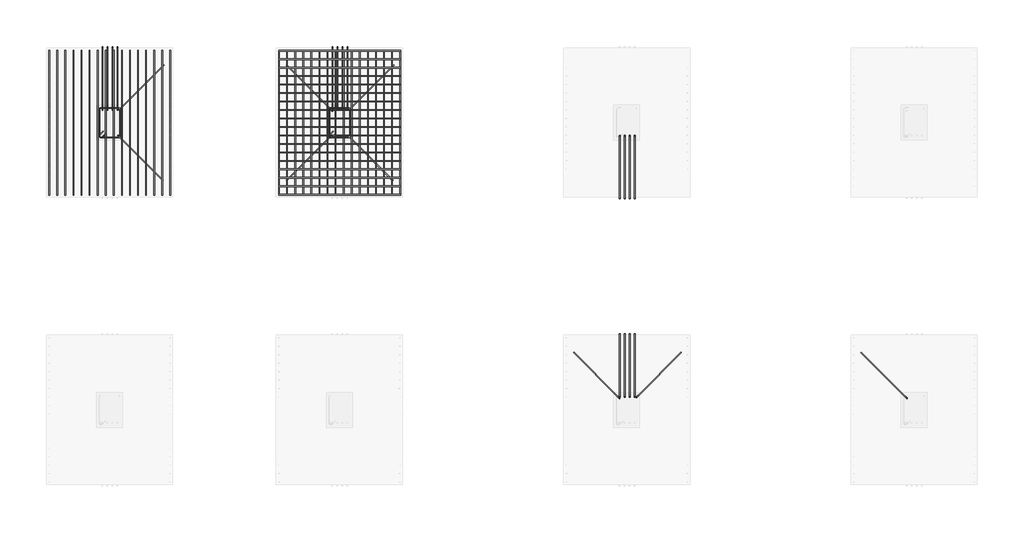
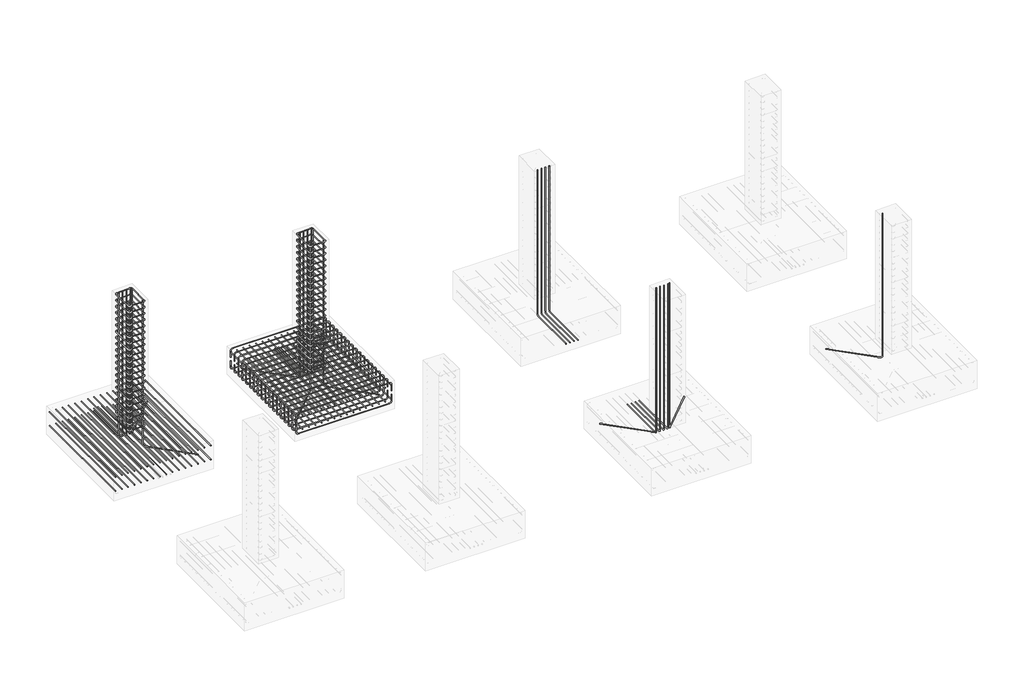
# One storey, part 5 of 33: 21 reinforcing bars.
"""IFC4 building model written with IfcOpenShell, lengths in millimetres."""

from ifc_helpers import new_model, si_unit, point, frame, origin, place, context, project, spatial, polyline, circle_curve, trimmed, segment, composite_curve, source, transform, mapped, element, save
from ifc_brep_helpers import swept_disk

model = new_model("IFC4")

# Units and contexts
model_context = context("Model", 3, world=origin())
ifc_project = project(units=[si_unit("LENGTHUNIT", "METRE", prefix="MILLI")], contexts=[model_context])

# Site, building, storey
site = spatial("IfcSite", under=ifc_project)
building = spatial("IfcBuilding", under=site)
storey = spatial("IfcBuildingStorey", under=building, Elevation=-3000.0)

# Reinforcing bars
placement = place(None, origin())
reinforcing_bar_shape = source(origin(), model_context, "Body", "SolidModel", [
    swept_disk(composite_curve([segment(polyline([(-10693.4642742, -2044.0608134, -3240.0), (-10693.4642742, -2044.0608134, -3092.7)]), True, "CONTINUOUS"), segment(trimmed(circle_curve(frame((-10647.1142742, -2044.0608134, -3092.7), z_axis=(0.0, 1.0, 0.0), x_axis=(-46.350000000000364, 0.0, 0.0)), 46.35), [point((-10693.4642742, -2044.0608134, -3092.7))], [point((-10647.1142742, -2044.0608134, -3046.35))], True, "CARTESIAN"), True, "CONTINUOUS"), segment(polyline([(-10647.1142742, -2044.0608134, -3046.35), (-8632.5142742, -2044.0608134, -3046.35)]), True, "CONTINUOUS"), segment(trimmed(circle_curve(frame((-8632.5142742, -2044.0608134, -3092.7), z_axis=(0.0, 1.0, 0.0), x_axis=(0.0, 0.0, 46.34999999999991)), 46.35), [point((-8632.5142742, -2044.0608134, -3046.35))], [point((-8586.1642742, -2044.0608134, -3092.7))], True, "CARTESIAN"), True, "CONTINUOUS"), segment(polyline([(-8586.1642742, -2044.0608134, -3092.7), (-8586.1642742, -2044.0608134, -3240.0)]), True, "CONTINUOUS")], self_intersect=False), 6.35),
])
element("IfcReinforcingBar", 1, at=placement, inside=storey, context=model_context, shape_type="MappedRepresentation", body=[
    mapped(reinforcing_bar_shape, transform((0.0, 0.0, 0.0), x_axis=(1.0, 0.0, 0.0), y_axis=(0.0, 1.0, 0.0), z_axis=(0.0, 0.0, 1.0))),
    mapped(reinforcing_bar_shape, transform((0.0, -147.4882353, 0.0), x_axis=(1.0, 0.0, 0.0), y_axis=(0.0, 1.0, 0.0), z_axis=(0.0, 0.0, 1.0))),
    mapped(reinforcing_bar_shape, transform((0.0, -294.9764706, 0.0), x_axis=(1.0, 0.0, 0.0), y_axis=(0.0, 1.0, 0.0), z_axis=(0.0, 0.0, 1.0))),
    mapped(reinforcing_bar_shape, transform((0.0, -442.4647059, 0.0), x_axis=(1.0, 0.0, 0.0), y_axis=(0.0, 1.0, 0.0), z_axis=(0.0, 0.0, 1.0))),
    mapped(reinforcing_bar_shape, transform((0.0, -589.9529412, 0.0), x_axis=(1.0, 0.0, 0.0), y_axis=(0.0, 1.0, 0.0), z_axis=(0.0, 0.0, 1.0))),
    mapped(reinforcing_bar_shape, transform((0.0, -737.4411765, 0.0), x_axis=(1.0, 0.0, 0.0), y_axis=(0.0, 1.0, 0.0), z_axis=(0.0, 0.0, 1.0))),
    mapped(reinforcing_bar_shape, transform((0.0, -884.9294118, 0.0), x_axis=(1.0, 0.0, 0.0), y_axis=(0.0, 1.0, 0.0), z_axis=(0.0, 0.0, 1.0))),
    mapped(reinforcing_bar_shape, transform((0.0, -1032.4176471, 0.0), x_axis=(1.0, 0.0, 0.0), y_axis=(0.0, 1.0, 0.0), z_axis=(0.0, 0.0, 1.0))),
    mapped(reinforcing_bar_shape, transform((0.0, -1179.9058824, 0.0), x_axis=(1.0, 0.0, 0.0), y_axis=(0.0, 1.0, 0.0), z_axis=(0.0, 0.0, 1.0))),
    mapped(reinforcing_bar_shape, transform((0.0, -1327.3941176, 0.0), x_axis=(1.0, 0.0, 0.0), y_axis=(0.0, 1.0, 0.0), z_axis=(0.0, 0.0, 1.0))),
    mapped(reinforcing_bar_shape, transform((0.0, -1474.8823529, 0.0), x_axis=(1.0, 0.0, 0.0), y_axis=(0.0, 1.0, 0.0), z_axis=(0.0, 0.0, 1.0))),
    mapped(reinforcing_bar_shape, transform((0.0, -1622.3705882, 0.0), x_axis=(1.0, 0.0, 0.0), y_axis=(0.0, 1.0, 0.0), z_axis=(0.0, 0.0, 1.0))),
    mapped(reinforcing_bar_shape, transform((0.0, -1769.8588235, 0.0), x_axis=(1.0, 0.0, 0.0), y_axis=(0.0, 1.0, 0.0), z_axis=(0.0, 0.0, 1.0))),
    mapped(reinforcing_bar_shape, transform((0.0, -1917.3470588, 0.0), x_axis=(1.0, 0.0, 0.0), y_axis=(0.0, 1.0, 0.0), z_axis=(0.0, 0.0, 1.0))),
    mapped(reinforcing_bar_shape, transform((0.0, -2064.8352941, 0.0), x_axis=(1.0, 0.0, 0.0), y_axis=(0.0, 1.0, 0.0), z_axis=(0.0, 0.0, 1.0))),
    mapped(reinforcing_bar_shape, transform((0.0, -2212.3235294, 0.0), x_axis=(1.0, 0.0, 0.0), y_axis=(0.0, 1.0, 0.0), z_axis=(0.0, 0.0, 1.0))),
    mapped(reinforcing_bar_shape, transform((0.0, -2359.8117647, 0.0), x_axis=(1.0, 0.0, 0.0), y_axis=(0.0, 1.0, 0.0), z_axis=(0.0, 0.0, 1.0))),
    mapped(reinforcing_bar_shape, transform((0.0, -2507.3, 0.0), x_axis=(1.0, 0.0, 0.0), y_axis=(0.0, 1.0, 0.0), z_axis=(0.0, 0.0, 1.0))),
])
reinforcing_bar_2_shape = source(origin(), model_context, "Body", "SolidModel", [
    swept_disk(composite_curve([segment(polyline([(-8586.1642742, -2044.0608134, -3330.080452), (-8586.1642742, -2044.0608134, -3477.380452)]), True, "CONTINUOUS"), segment(trimmed(circle_curve(frame((-8632.5142742, -2044.0608134, -3477.380452), z_axis=(0.0, 1.0, 0.0), x_axis=(46.350000000000364, 0.0, 0.0)), 46.35), [point((-8586.1642742, -2044.0608134, -3477.380452))], [point((-8632.5142742, -2044.0608134, -3523.730452))], True, "CARTESIAN"), True, "CONTINUOUS"), segment(polyline([(-8632.5142742, -2044.0608134, -3523.730452), (-10647.1142742, -2044.0608134, -3523.730452)]), True, "CONTINUOUS"), segment(trimmed(circle_curve(frame((-10647.1142742, -2044.0608134, -3477.380452), z_axis=(0.0, 1.0, 0.0), x_axis=(0.0, 0.0, -46.34999999999991)), 46.35), [point((-10647.1142742, -2044.0608134, -3523.730452))], [point((-10693.4642742, -2044.0608134, -3477.380452))], True, "CARTESIAN"), True, "CONTINUOUS"), segment(polyline([(-10693.4642742, -2044.0608134, -3477.380452), (-10693.4642742, -2044.0608134, -3330.080452)]), True, "CONTINUOUS")], self_intersect=False), 6.35),
])
element("IfcReinforcingBar", 2, at=placement, inside=storey, context=model_context, shape_type="MappedRepresentation", body=[
    mapped(reinforcing_bar_2_shape, transform((0.0, 0.0, 0.0), x_axis=(1.0, 0.0, 0.0), y_axis=(0.0, 1.0, 0.0), z_axis=(0.0, 0.0, 1.0))),
    mapped(reinforcing_bar_2_shape, transform((0.0, -147.4882353, 0.0), x_axis=(1.0, 0.0, 0.0), y_axis=(0.0, 1.0, 0.0), z_axis=(0.0, 0.0, 1.0))),
    mapped(reinforcing_bar_2_shape, transform((0.0, -294.9764706, 0.0), x_axis=(1.0, 0.0, 0.0), y_axis=(0.0, 1.0, 0.0), z_axis=(0.0, 0.0, 1.0))),
    mapped(reinforcing_bar_2_shape, transform((0.0, -442.4647059, 0.0), x_axis=(1.0, 0.0, 0.0), y_axis=(0.0, 1.0, 0.0), z_axis=(0.0, 0.0, 1.0))),
    mapped(reinforcing_bar_2_shape, transform((0.0, -589.9529412, 0.0), x_axis=(1.0, 0.0, 0.0), y_axis=(0.0, 1.0, 0.0), z_axis=(0.0, 0.0, 1.0))),
    mapped(reinforcing_bar_2_shape, transform((0.0, -737.4411765, 0.0), x_axis=(1.0, 0.0, 0.0), y_axis=(0.0, 1.0, 0.0), z_axis=(0.0, 0.0, 1.0))),
    mapped(reinforcing_bar_2_shape, transform((0.0, -884.9294118, 0.0), x_axis=(1.0, 0.0, 0.0), y_axis=(0.0, 1.0, 0.0), z_axis=(0.0, 0.0, 1.0))),
    mapped(reinforcing_bar_2_shape, transform((0.0, -1032.4176471, 0.0), x_axis=(1.0, 0.0, 0.0), y_axis=(0.0, 1.0, 0.0), z_axis=(0.0, 0.0, 1.0))),
    mapped(reinforcing_bar_2_shape, transform((0.0, -1179.9058824, 0.0), x_axis=(1.0, 0.0, 0.0), y_axis=(0.0, 1.0, 0.0), z_axis=(0.0, 0.0, 1.0))),
    mapped(reinforcing_bar_2_shape, transform((0.0, -1327.3941176, 0.0), x_axis=(1.0, 0.0, 0.0), y_axis=(0.0, 1.0, 0.0), z_axis=(0.0, 0.0, 1.0))),
    mapped(reinforcing_bar_2_shape, transform((0.0, -1474.8823529, 0.0), x_axis=(1.0, 0.0, 0.0), y_axis=(0.0, 1.0, 0.0), z_axis=(0.0, 0.0, 1.0))),
    mapped(reinforcing_bar_2_shape, transform((0.0, -1622.3705882, 0.0), x_axis=(1.0, 0.0, 0.0), y_axis=(0.0, 1.0, 0.0), z_axis=(0.0, 0.0, 1.0))),
    mapped(reinforcing_bar_2_shape, transform((0.0, -1769.8588235, 0.0), x_axis=(1.0, 0.0, 0.0), y_axis=(0.0, 1.0, 0.0), z_axis=(0.0, 0.0, 1.0))),
    mapped(reinforcing_bar_2_shape, transform((0.0, -1917.3470588, 0.0), x_axis=(1.0, 0.0, 0.0), y_axis=(0.0, 1.0, 0.0), z_axis=(0.0, 0.0, 1.0))),
    mapped(reinforcing_bar_2_shape, transform((0.0, -2064.8352941, 0.0), x_axis=(1.0, 0.0, 0.0), y_axis=(0.0, 1.0, 0.0), z_axis=(0.0, 0.0, 1.0))),
    mapped(reinforcing_bar_2_shape, transform((0.0, -2212.3235294, 0.0), x_axis=(1.0, 0.0, 0.0), y_axis=(0.0, 1.0, 0.0), z_axis=(0.0, 0.0, 1.0))),
    mapped(reinforcing_bar_2_shape, transform((0.0, -2359.8117647, 0.0), x_axis=(1.0, 0.0, 0.0), y_axis=(0.0, 1.0, 0.0), z_axis=(0.0, 0.0, 1.0))),
    mapped(reinforcing_bar_2_shape, transform((0.0, -2507.3, 0.0), x_axis=(1.0, 0.0, 0.0), y_axis=(0.0, 1.0, 0.0), z_axis=(0.0, 0.0, 1.0))),
])
reinforcing_bar_3_shape = source(origin(), model_context, "Body", "SolidModel", [
    swept_disk(composite_curve([segment(polyline([(-8586.1642742, -4557.7108134, -3447.8614173), (-8586.1642742, -2037.7108134, -3447.8614173)]), True, "CONTINUOUS")], self_intersect=False), 6.35),
])
element("IfcReinforcingBar", 3, at=placement, inside=storey, context=model_context, shape_type="MappedRepresentation", body=[
    mapped(reinforcing_bar_3_shape, transform((0.0, 0.0, 0.0), x_axis=(1.0, 0.0, 0.0), y_axis=(0.0, 1.0, 0.0), z_axis=(0.0, 0.0, 1.0))),
    mapped(reinforcing_bar_3_shape, transform((-140.4866667, 0.0, 0.0), x_axis=(1.0, 0.0, 0.0), y_axis=(0.0, 1.0, 0.0), z_axis=(0.0, 0.0, 1.0))),
    mapped(reinforcing_bar_3_shape, transform((-280.9733333, 0.0, 0.0), x_axis=(1.0, 0.0, 0.0), y_axis=(0.0, 1.0, 0.0), z_axis=(0.0, 0.0, 1.0))),
    mapped(reinforcing_bar_3_shape, transform((-421.46, 0.0, 0.0), x_axis=(1.0, 0.0, 0.0), y_axis=(0.0, 1.0, 0.0), z_axis=(0.0, 0.0, 1.0))),
    mapped(reinforcing_bar_3_shape, transform((-561.9466667, 0.0, 0.0), x_axis=(1.0, 0.0, 0.0), y_axis=(0.0, 1.0, 0.0), z_axis=(0.0, 0.0, 1.0))),
    mapped(reinforcing_bar_3_shape, transform((-702.4333333, 0.0, 0.0), x_axis=(1.0, 0.0, 0.0), y_axis=(0.0, 1.0, 0.0), z_axis=(0.0, 0.0, 1.0))),
    mapped(reinforcing_bar_3_shape, transform((-842.92, 0.0, 0.0), x_axis=(1.0, 0.0, 0.0), y_axis=(0.0, 1.0, 0.0), z_axis=(0.0, 0.0, 1.0))),
    mapped(reinforcing_bar_3_shape, transform((-983.4066667, 0.0, 0.0), x_axis=(1.0, 0.0, 0.0), y_axis=(0.0, 1.0, 0.0), z_axis=(0.0, 0.0, 1.0))),
    mapped(reinforcing_bar_3_shape, transform((-1123.8933333, 0.0, 0.0), x_axis=(1.0, 0.0, 0.0), y_axis=(0.0, 1.0, 0.0), z_axis=(0.0, 0.0, 1.0))),
    mapped(reinforcing_bar_3_shape, transform((-1264.38, 0.0, 0.0), x_axis=(1.0, 0.0, 0.0), y_axis=(0.0, 1.0, 0.0), z_axis=(0.0, 0.0, 1.0))),
    mapped(reinforcing_bar_3_shape, transform((-1404.8666667, 0.0, 0.0), x_axis=(1.0, 0.0, 0.0), y_axis=(0.0, 1.0, 0.0), z_axis=(0.0, 0.0, 1.0))),
    mapped(reinforcing_bar_3_shape, transform((-1545.3533333, 0.0, 0.0), x_axis=(1.0, 0.0, 0.0), y_axis=(0.0, 1.0, 0.0), z_axis=(0.0, 0.0, 1.0))),
    mapped(reinforcing_bar_3_shape, transform((-1685.84, 0.0, 0.0), x_axis=(1.0, 0.0, 0.0), y_axis=(0.0, 1.0, 0.0), z_axis=(0.0, 0.0, 1.0))),
    mapped(reinforcing_bar_3_shape, transform((-1826.3266667, 0.0, 0.0), x_axis=(1.0, 0.0, 0.0), y_axis=(0.0, 1.0, 0.0), z_axis=(0.0, 0.0, 1.0))),
    mapped(reinforcing_bar_3_shape, transform((-1966.8133333, 0.0, 0.0), x_axis=(1.0, 0.0, 0.0), y_axis=(0.0, 1.0, 0.0), z_axis=(0.0, 0.0, 1.0))),
    mapped(reinforcing_bar_3_shape, transform((-2107.3, 0.0, 0.0), x_axis=(1.0, 0.0, 0.0), y_axis=(0.0, 1.0, 0.0), z_axis=(0.0, 0.0, 1.0))),
])
reinforcing_bar_4_shape = source(origin(), model_context, "Body", "SolidModel", [
    swept_disk(composite_curve([segment(polyline([(-10693.4642742, -4557.7108134, -3122.7084113), (-10693.4642742, -2037.7108134, -3122.7084113)]), True, "CONTINUOUS")], self_intersect=False), 6.35),
])
element("IfcReinforcingBar", 4, at=placement, inside=storey, context=model_context, shape_type="MappedRepresentation", body=[
    mapped(reinforcing_bar_4_shape, transform((0.0, 0.0, 0.0), x_axis=(1.0, 0.0, 0.0), y_axis=(0.0, 1.0, 0.0), z_axis=(0.0, 0.0, 1.0))),
    mapped(reinforcing_bar_4_shape, transform((140.4866667, 0.0, 0.0), x_axis=(1.0, 0.0, 0.0), y_axis=(0.0, 1.0, 0.0), z_axis=(0.0, 0.0, 1.0))),
    mapped(reinforcing_bar_4_shape, transform((280.9733333, 0.0, 0.0), x_axis=(1.0, 0.0, 0.0), y_axis=(0.0, 1.0, 0.0), z_axis=(0.0, 0.0, 1.0))),
    mapped(reinforcing_bar_4_shape, transform((421.46, 0.0, 0.0), x_axis=(1.0, 0.0, 0.0), y_axis=(0.0, 1.0, 0.0), z_axis=(0.0, 0.0, 1.0))),
    mapped(reinforcing_bar_4_shape, transform((561.9466667, 0.0, 0.0), x_axis=(1.0, 0.0, 0.0), y_axis=(0.0, 1.0, 0.0), z_axis=(0.0, 0.0, 1.0))),
    mapped(reinforcing_bar_4_shape, transform((702.4333333, 0.0, 0.0), x_axis=(1.0, 0.0, 0.0), y_axis=(0.0, 1.0, 0.0), z_axis=(0.0, 0.0, 1.0))),
    mapped(reinforcing_bar_4_shape, transform((842.92, 0.0, 0.0), x_axis=(1.0, 0.0, 0.0), y_axis=(0.0, 1.0, 0.0), z_axis=(0.0, 0.0, 1.0))),
    mapped(reinforcing_bar_4_shape, transform((983.4066667, 0.0, 0.0), x_axis=(1.0, 0.0, 0.0), y_axis=(0.0, 1.0, 0.0), z_axis=(0.0, 0.0, 1.0))),
    mapped(reinforcing_bar_4_shape, transform((1123.8933333, 0.0, 0.0), x_axis=(1.0, 0.0, 0.0), y_axis=(0.0, 1.0, 0.0), z_axis=(0.0, 0.0, 1.0))),
    mapped(reinforcing_bar_4_shape, transform((1264.38, 0.0, 0.0), x_axis=(1.0, 0.0, 0.0), y_axis=(0.0, 1.0, 0.0), z_axis=(0.0, 0.0, 1.0))),
    mapped(reinforcing_bar_4_shape, transform((1404.8666667, 0.0, 0.0), x_axis=(1.0, 0.0, 0.0), y_axis=(0.0, 1.0, 0.0), z_axis=(0.0, 0.0, 1.0))),
    mapped(reinforcing_bar_4_shape, transform((1545.3533333, 0.0, 0.0), x_axis=(1.0, 0.0, 0.0), y_axis=(0.0, 1.0, 0.0), z_axis=(0.0, 0.0, 1.0))),
    mapped(reinforcing_bar_4_shape, transform((1685.84, 0.0, 0.0), x_axis=(1.0, 0.0, 0.0), y_axis=(0.0, 1.0, 0.0), z_axis=(0.0, 0.0, 1.0))),
    mapped(reinforcing_bar_4_shape, transform((1826.3266667, 0.0, 0.0), x_axis=(1.0, 0.0, 0.0), y_axis=(0.0, 1.0, 0.0), z_axis=(0.0, 0.0, 1.0))),
    mapped(reinforcing_bar_4_shape, transform((1966.8133333, 0.0, 0.0), x_axis=(1.0, 0.0, 0.0), y_axis=(0.0, 1.0, 0.0), z_axis=(0.0, 0.0, 1.0))),
    mapped(reinforcing_bar_4_shape, transform((2107.3, 0.0, 0.0), x_axis=(1.0, 0.0, 0.0), y_axis=(0.0, 1.0, 0.0), z_axis=(0.0, 0.0, 1.0))),
])
reinforcing_bar_5_shape = source(origin(), model_context, "Body", "SolidModel", [
    swept_disk(composite_curve([segment(polyline([(-12586.1642742, -4557.7108134, -3447.8614173), (-12586.1642742, -2037.7108134, -3447.8614173)]), True, "CONTINUOUS")], self_intersect=False), 6.35),
])
element("IfcReinforcingBar", 5, at=placement, inside=storey, context=model_context, shape_type="MappedRepresentation", body=[
    mapped(reinforcing_bar_5_shape, transform((0.0, 0.0, 0.0), x_axis=(1.0, 0.0, 0.0), y_axis=(0.0, 1.0, 0.0), z_axis=(0.0, 0.0, 1.0))),
    mapped(reinforcing_bar_5_shape, transform((-140.4866667, 0.0, 0.0), x_axis=(1.0, 0.0, 0.0), y_axis=(0.0, 1.0, 0.0), z_axis=(0.0, 0.0, 1.0))),
    mapped(reinforcing_bar_5_shape, transform((-280.9733333, 0.0, 0.0), x_axis=(1.0, 0.0, 0.0), y_axis=(0.0, 1.0, 0.0), z_axis=(0.0, 0.0, 1.0))),
    mapped(reinforcing_bar_5_shape, transform((-421.46, 0.0, 0.0), x_axis=(1.0, 0.0, 0.0), y_axis=(0.0, 1.0, 0.0), z_axis=(0.0, 0.0, 1.0))),
    mapped(reinforcing_bar_5_shape, transform((-561.9466667, 0.0, 0.0), x_axis=(1.0, 0.0, 0.0), y_axis=(0.0, 1.0, 0.0), z_axis=(0.0, 0.0, 1.0))),
    mapped(reinforcing_bar_5_shape, transform((-702.4333333, 0.0, 0.0), x_axis=(1.0, 0.0, 0.0), y_axis=(0.0, 1.0, 0.0), z_axis=(0.0, 0.0, 1.0))),
    mapped(reinforcing_bar_5_shape, transform((-842.92, 0.0, 0.0), x_axis=(1.0, 0.0, 0.0), y_axis=(0.0, 1.0, 0.0), z_axis=(0.0, 0.0, 1.0))),
    mapped(reinforcing_bar_5_shape, transform((-983.4066667, 0.0, 0.0), x_axis=(1.0, 0.0, 0.0), y_axis=(0.0, 1.0, 0.0), z_axis=(0.0, 0.0, 1.0))),
    mapped(reinforcing_bar_5_shape, transform((-1123.8933333, 0.0, 0.0), x_axis=(1.0, 0.0, 0.0), y_axis=(0.0, 1.0, 0.0), z_axis=(0.0, 0.0, 1.0))),
    mapped(reinforcing_bar_5_shape, transform((-1264.38, 0.0, 0.0), x_axis=(1.0, 0.0, 0.0), y_axis=(0.0, 1.0, 0.0), z_axis=(0.0, 0.0, 1.0))),
    mapped(reinforcing_bar_5_shape, transform((-1404.8666667, 0.0, 0.0), x_axis=(1.0, 0.0, 0.0), y_axis=(0.0, 1.0, 0.0), z_axis=(0.0, 0.0, 1.0))),
    mapped(reinforcing_bar_5_shape, transform((-1545.3533333, 0.0, 0.0), x_axis=(1.0, 0.0, 0.0), y_axis=(0.0, 1.0, 0.0), z_axis=(0.0, 0.0, 1.0))),
    mapped(reinforcing_bar_5_shape, transform((-1685.84, 0.0, 0.0), x_axis=(1.0, 0.0, 0.0), y_axis=(0.0, 1.0, 0.0), z_axis=(0.0, 0.0, 1.0))),
    mapped(reinforcing_bar_5_shape, transform((-1826.3266667, 0.0, 0.0), x_axis=(1.0, 0.0, 0.0), y_axis=(0.0, 1.0, 0.0), z_axis=(0.0, 0.0, 1.0))),
    mapped(reinforcing_bar_5_shape, transform((-1966.8133333, 0.0, 0.0), x_axis=(1.0, 0.0, 0.0), y_axis=(0.0, 1.0, 0.0), z_axis=(0.0, 0.0, 1.0))),
    mapped(reinforcing_bar_5_shape, transform((-2107.3, 0.0, 0.0), x_axis=(1.0, 0.0, 0.0), y_axis=(0.0, 1.0, 0.0), z_axis=(0.0, 0.0, 1.0))),
])
reinforcing_bar_6_shape = source(origin(), model_context, "Body", "SolidModel", [
    swept_disk(composite_curve([segment(polyline([(-14693.4642742, -4557.7108134, -3122.7084113), (-14693.4642742, -2037.7108134, -3122.7084113)]), True, "CONTINUOUS")], self_intersect=False), 6.35),
])
element("IfcReinforcingBar", 6, at=placement, inside=storey, context=model_context, shape_type="MappedRepresentation", body=[
    mapped(reinforcing_bar_6_shape, transform((0.0, 0.0, 0.0), x_axis=(1.0, 0.0, 0.0), y_axis=(0.0, 1.0, 0.0), z_axis=(0.0, 0.0, 1.0))),
    mapped(reinforcing_bar_6_shape, transform((140.4866667, 0.0, 0.0), x_axis=(1.0, 0.0, 0.0), y_axis=(0.0, 1.0, 0.0), z_axis=(0.0, 0.0, 1.0))),
    mapped(reinforcing_bar_6_shape, transform((280.9733333, 0.0, 0.0), x_axis=(1.0, 0.0, 0.0), y_axis=(0.0, 1.0, 0.0), z_axis=(0.0, 0.0, 1.0))),
    mapped(reinforcing_bar_6_shape, transform((421.46, 0.0, 0.0), x_axis=(1.0, 0.0, 0.0), y_axis=(0.0, 1.0, 0.0), z_axis=(0.0, 0.0, 1.0))),
    mapped(reinforcing_bar_6_shape, transform((561.9466667, 0.0, 0.0), x_axis=(1.0, 0.0, 0.0), y_axis=(0.0, 1.0, 0.0), z_axis=(0.0, 0.0, 1.0))),
    mapped(reinforcing_bar_6_shape, transform((702.4333333, 0.0, 0.0), x_axis=(1.0, 0.0, 0.0), y_axis=(0.0, 1.0, 0.0), z_axis=(0.0, 0.0, 1.0))),
    mapped(reinforcing_bar_6_shape, transform((842.92, 0.0, 0.0), x_axis=(1.0, 0.0, 0.0), y_axis=(0.0, 1.0, 0.0), z_axis=(0.0, 0.0, 1.0))),
    mapped(reinforcing_bar_6_shape, transform((983.4066667, 0.0, 0.0), x_axis=(1.0, 0.0, 0.0), y_axis=(0.0, 1.0, 0.0), z_axis=(0.0, 0.0, 1.0))),
    mapped(reinforcing_bar_6_shape, transform((1123.8933333, 0.0, 0.0), x_axis=(1.0, 0.0, 0.0), y_axis=(0.0, 1.0, 0.0), z_axis=(0.0, 0.0, 1.0))),
    mapped(reinforcing_bar_6_shape, transform((1264.38, 0.0, 0.0), x_axis=(1.0, 0.0, 0.0), y_axis=(0.0, 1.0, 0.0), z_axis=(0.0, 0.0, 1.0))),
    mapped(reinforcing_bar_6_shape, transform((1404.8666667, 0.0, 0.0), x_axis=(1.0, 0.0, 0.0), y_axis=(0.0, 1.0, 0.0), z_axis=(0.0, 0.0, 1.0))),
    mapped(reinforcing_bar_6_shape, transform((1545.3533333, 0.0, 0.0), x_axis=(1.0, 0.0, 0.0), y_axis=(0.0, 1.0, 0.0), z_axis=(0.0, 0.0, 1.0))),
    mapped(reinforcing_bar_6_shape, transform((1685.84, 0.0, 0.0), x_axis=(1.0, 0.0, 0.0), y_axis=(0.0, 1.0, 0.0), z_axis=(0.0, 0.0, 1.0))),
    mapped(reinforcing_bar_6_shape, transform((1826.3266667, 0.0, 0.0), x_axis=(1.0, 0.0, 0.0), y_axis=(0.0, 1.0, 0.0), z_axis=(0.0, 0.0, 1.0))),
    mapped(reinforcing_bar_6_shape, transform((1966.8133333, 0.0, 0.0), x_axis=(1.0, 0.0, 0.0), y_axis=(0.0, 1.0, 0.0), z_axis=(0.0, 0.0, 1.0))),
    mapped(reinforcing_bar_6_shape, transform((2107.3, 0.0, 0.0), x_axis=(1.0, 0.0, 0.0), y_axis=(0.0, 1.0, 0.0), z_axis=(0.0, 0.0, 1.0))),
])
reinforcing_bar_7_shape = source(origin(), model_context, "Body", "SolidModel", [
    swept_disk(composite_curve([segment(polyline([(-13753.5385089, -3446.8994528, -2953.65), (-13809.2820718, -3502.6430158, -2953.65)]), True, "CONTINUOUS"), segment(trimmed(circle_curve(frame((-13787.1142742, -3524.8108134, -2953.65), z_axis=(0.0, 0.0, 1.0), x_axis=(-22.167797600000995, 22.167797600000085, 0.0)), 31.35), [point((-13809.2820718, -3502.6430158, -2953.65))], [point((-13787.1142742, -3556.1608134, -2953.65))], True, "CARTESIAN"), True, "CONTINUOUS"), segment(polyline([(-13787.1142742, -3556.1608134, -2953.65), (-13492.5142742, -3556.1608134, -2953.65)]), True, "CONTINUOUS"), segment(trimmed(circle_curve(frame((-13492.5142742, -3524.8108134, -2953.65), z_axis=(0.0, 0.0, 1.0), x_axis=(0.0, -31.34999999999991, 0.0)), 31.35), [point((-13492.5142742, -3556.1608134, -2953.65))], [point((-13461.1642742, -3524.8108134, -2953.65))], True, "CARTESIAN"), True, "CONTINUOUS"), segment(polyline([(-13461.1642742, -3524.8108134, -2953.65), (-13461.1642742, -3070.6108134, -2953.65)]), True, "CONTINUOUS"), segment(trimmed(circle_curve(frame((-13492.4944891, -3070.6108134, -2954.7636125), z_axis=(-0.0355219283344822, 0.0, 0.9993688971583016), x_axis=(31.33021489999919, 0.0, 1.1136124999998174)), 31.35), [point((-13461.1642742, -3070.6108134, -2953.65))], [point((-13492.4944891, -3039.2608134, -2954.7636125))], True, "CARTESIAN"), True, "CONTINUOUS"), segment(polyline([(-13492.4944891, -3039.2608134, -2954.7636125), (-13787.1340593, -3039.2608134, -2965.2363875)]), True, "CONTINUOUS"), segment(trimmed(circle_curve(frame((-13787.1340593, -3070.6108134, -2965.2363875), z_axis=(-0.0355219283344822, 0.0, 0.9993688971583016), x_axis=(0.0, 31.34999999999991, 0.0)), 31.35), [point((-13787.1340593, -3039.2608134, -2965.2363875))], [point((-13818.4642742, -3070.6108134, -2966.35))], True, "CARTESIAN"), True, "CONTINUOUS"), segment(polyline([(-13818.4642742, -3070.6108134, -2966.35), (-13818.4642742, -3524.8108134, -2966.35)]), True, "CONTINUOUS"), segment(trimmed(circle_curve(frame((-13787.1142742, -3524.8108134, -2966.35), z_axis=(0.0, 0.0, 1.0), x_axis=(-31.350000000000364, 0.0, 0.0)), 31.35), [point((-13818.4642742, -3524.8108134, -2966.35))], [point((-13764.9464766, -3546.978611, -2966.35))], True, "CARTESIAN"), True, "CONTINUOUS"), segment(polyline([(-13764.9464766, -3546.978611, -2966.35), (-13709.2029137, -3491.235048, -2966.35)]), True, "CONTINUOUS")], self_intersect=False), 6.35),
])
element("IfcReinforcingBar", 7, at=placement, inside=storey, context=model_context, shape_type="MappedRepresentation", body=[
    mapped(reinforcing_bar_7_shape, transform((0.0, 0.0, 0.0), x_axis=(1.0, 0.0, 0.0), y_axis=(0.0, 1.0, 0.0), z_axis=(0.0, 0.0, 1.0))),
    mapped(reinforcing_bar_7_shape, transform((0.0, 0.0, 145.365), x_axis=(1.0, 0.0, 0.0), y_axis=(0.0, 1.0, 0.0), z_axis=(0.0, 0.0, 1.0))),
    mapped(reinforcing_bar_7_shape, transform((0.0, 0.0, 290.73), x_axis=(1.0, 0.0, 0.0), y_axis=(0.0, 1.0, 0.0), z_axis=(0.0, 0.0, 1.0))),
    mapped(reinforcing_bar_7_shape, transform((0.0, 0.0, 436.095), x_axis=(1.0, 0.0, 0.0), y_axis=(0.0, 1.0, 0.0), z_axis=(0.0, 0.0, 1.0))),
    mapped(reinforcing_bar_7_shape, transform((0.0, 0.0, 581.46), x_axis=(1.0, 0.0, 0.0), y_axis=(0.0, 1.0, 0.0), z_axis=(0.0, 0.0, 1.0))),
    mapped(reinforcing_bar_7_shape, transform((0.0, 0.0, 726.825), x_axis=(1.0, 0.0, 0.0), y_axis=(0.0, 1.0, 0.0), z_axis=(0.0, 0.0, 1.0))),
    mapped(reinforcing_bar_7_shape, transform((0.0, 0.0, 872.19), x_axis=(1.0, 0.0, 0.0), y_axis=(0.0, 1.0, 0.0), z_axis=(0.0, 0.0, 1.0))),
    mapped(reinforcing_bar_7_shape, transform((0.0, 0.0, 1017.555), x_axis=(1.0, 0.0, 0.0), y_axis=(0.0, 1.0, 0.0), z_axis=(0.0, 0.0, 1.0))),
    mapped(reinforcing_bar_7_shape, transform((0.0, 0.0, 1162.92), x_axis=(1.0, 0.0, 0.0), y_axis=(0.0, 1.0, 0.0), z_axis=(0.0, 0.0, 1.0))),
    mapped(reinforcing_bar_7_shape, transform((0.0, 0.0, 1308.285), x_axis=(1.0, 0.0, 0.0), y_axis=(0.0, 1.0, 0.0), z_axis=(0.0, 0.0, 1.0))),
    mapped(reinforcing_bar_7_shape, transform((0.0, 0.0, 1453.65), x_axis=(1.0, 0.0, 0.0), y_axis=(0.0, 1.0, 0.0), z_axis=(0.0, 0.0, 1.0))),
    mapped(reinforcing_bar_7_shape, transform((0.0, 0.0, 1599.015), x_axis=(1.0, 0.0, 0.0), y_axis=(0.0, 1.0, 0.0), z_axis=(0.0, 0.0, 1.0))),
    mapped(reinforcing_bar_7_shape, transform((0.0, 0.0, 1744.38), x_axis=(1.0, 0.0, 0.0), y_axis=(0.0, 1.0, 0.0), z_axis=(0.0, 0.0, 1.0))),
    mapped(reinforcing_bar_7_shape, transform((0.0, 0.0, 1889.745), x_axis=(1.0, 0.0, 0.0), y_axis=(0.0, 1.0, 0.0), z_axis=(0.0, 0.0, 1.0))),
    mapped(reinforcing_bar_7_shape, transform((0.0, 0.0, 2035.11), x_axis=(1.0, 0.0, 0.0), y_axis=(0.0, 1.0, 0.0), z_axis=(0.0, 0.0, 1.0))),
    mapped(reinforcing_bar_7_shape, transform((0.0, 0.0, 2180.475), x_axis=(1.0, 0.0, 0.0), y_axis=(0.0, 1.0, 0.0), z_axis=(0.0, 0.0, 1.0))),
    mapped(reinforcing_bar_7_shape, transform((0.0, 0.0, 2325.84), x_axis=(1.0, 0.0, 0.0), y_axis=(0.0, 1.0, 0.0), z_axis=(0.0, 0.0, 1.0))),
    mapped(reinforcing_bar_7_shape, transform((0.0, 0.0, 2471.205), x_axis=(1.0, 0.0, 0.0), y_axis=(0.0, 1.0, 0.0), z_axis=(0.0, 0.0, 1.0))),
    mapped(reinforcing_bar_7_shape, transform((0.0, 0.0, 2616.57), x_axis=(1.0, 0.0, 0.0), y_axis=(0.0, 1.0, 0.0), z_axis=(0.0, 0.0, 1.0))),
    mapped(reinforcing_bar_7_shape, transform((0.0, 0.0, 2761.935), x_axis=(1.0, 0.0, 0.0), y_axis=(0.0, 1.0, 0.0), z_axis=(0.0, 0.0, 1.0))),
    mapped(reinforcing_bar_7_shape, transform((0.0, 0.0, 2907.3), x_axis=(1.0, 0.0, 0.0), y_axis=(0.0, 1.0, 0.0), z_axis=(0.0, 0.0, 1.0))),
])
element("IfcReinforcingBar", 8, at=placement, inside=storey, context=model_context, shape_type="SolidModel", body=[
    swept_disk(composite_curve([segment(polyline([(-13492.8328699, -3521.6339414, -40.0), (-13492.8328699, -3521.6339414, -3393.65)]), True, "CONTINUOUS"), segment(trimmed(circle_curve(frame((-13460.0584706, -3554.4083407, -3393.65), z_axis=(-0.7071067811865493, -0.7071067811865459, 0.0), x_axis=(-32.77439929999855, 32.774399299999914, 0.0)), 46.35), [point((-13492.8328699, -3521.6339414, -3393.65))], [point((-13460.0584706, -3554.4083407, -3440.0))], True, "CARTESIAN"), True, "CONTINUOUS"), segment(polyline([(-13460.0584706, -3554.4083407, -3440.0), (-12715.0154106, -4299.4514007, -3440.0)]), True, "CONTINUOUS")], self_intersect=False), 6.35),
])
element("IfcReinforcingBar", 9, at=placement, inside=storey, context=model_context, shape_type="SolidModel", body=[
    swept_disk(composite_curve([segment(polyline([(-13474.2315783, -3073.7876853, -30.2564663), (-13474.2315783, -3073.7876853, -3383.9064663)]), True, "CONTINUOUS"), segment(trimmed(circle_curve(frame((-13441.457179, -3041.013286, -3383.9064663), z_axis=(0.7071067811865493, -0.7071067811865459, 0.0), x_axis=(-32.77439929999855, -32.774399299999914, 0.0)), 46.35), [point((-13474.2315783, -3073.7876853, -3383.9064663))], [point((-13441.457179, -3041.013286, -3430.2564663))], True, "CARTESIAN"), True, "CONTINUOUS"), segment(polyline([(-13441.457179, -3041.013286, -3430.2564663), (-12696.414119, -2295.970226, -3430.2564663)]), True, "CONTINUOUS")], self_intersect=False), 6.35),
])
reinforcing_bar_8_shape = source(origin(), model_context, "Body", "SolidModel", [
    swept_disk(composite_curve([segment(polyline([(-13763.8841678, -3071.9278134, -40.0), (-13763.8841678, -3071.9278134, -3393.65)]), True, "CONTINUOUS"), segment(trimmed(circle_curve(frame((-13763.8841678, -3025.5778134, -3393.65), z_axis=(1.0, 0.0, 0.0), x_axis=(0.0, -46.34999999999991, 0.0)), 46.35), [point((-13763.8841678, -3071.9278134, -3393.65))], [point((-13763.8841678, -3025.5778134, -3440.0))], True, "CARTESIAN"), True, "CONTINUOUS"), segment(polyline([(-13763.8841678, -3025.5778134, -3440.0), (-13763.8841678, -1971.9278134, -3440.0)]), True, "CONTINUOUS")], self_intersect=False), 6.35),
])
element("IfcReinforcingBar", 10, at=placement, inside=storey, context=model_context, shape_type="MappedRepresentation", body=[
    mapped(reinforcing_bar_8_shape, transform((0.0, 0.0, 0.0), x_axis=(1.0, 0.0, 0.0), y_axis=(0.0, 1.0, 0.0), z_axis=(0.0, 0.0, 1.0))),
    mapped(reinforcing_bar_8_shape, transform((86.8979716, 0.0, 0.0), x_axis=(1.0, 0.0, 0.0), y_axis=(0.0, 1.0, 0.0), z_axis=(0.0, 0.0, 1.0))),
    mapped(reinforcing_bar_8_shape, transform((173.7959432, 0.0, 0.0), x_axis=(1.0, 0.0, 0.0), y_axis=(0.0, 1.0, 0.0), z_axis=(0.0, 0.0, 1.0))),
    mapped(reinforcing_bar_8_shape, transform((260.6939148, 0.0, 0.0), x_axis=(1.0, 0.0, 0.0), y_axis=(0.0, 1.0, 0.0), z_axis=(0.0, 0.0, 1.0))),
])
reinforcing_bar_9_shape = source(origin(), model_context, "Body", "SolidModel", [
    swept_disk(composite_curve([segment(polyline([(-9753.5385089, -3446.8994528, -2953.65), (-9809.2820718, -3502.6430158, -2953.65)]), True, "CONTINUOUS"), segment(trimmed(circle_curve(frame((-9787.1142742, -3524.8108134, -2953.65), z_axis=(0.0, 0.0, 1.0), x_axis=(-22.167797600000995, 22.167797600000085, 0.0)), 31.35), [point((-9809.2820718, -3502.6430158, -2953.65))], [point((-9787.1142742, -3556.1608134, -2953.65))], True, "CARTESIAN"), True, "CONTINUOUS"), segment(polyline([(-9787.1142742, -3556.1608134, -2953.65), (-9492.5142742, -3556.1608134, -2953.65)]), True, "CONTINUOUS"), segment(trimmed(circle_curve(frame((-9492.5142742, -3524.8108134, -2953.65), z_axis=(0.0, 0.0, 1.0), x_axis=(0.0, -31.34999999999991, 0.0)), 31.35), [point((-9492.5142742, -3556.1608134, -2953.65))], [point((-9461.1642742, -3524.8108134, -2953.65))], True, "CARTESIAN"), True, "CONTINUOUS"), segment(polyline([(-9461.1642742, -3524.8108134, -2953.65), (-9461.1642742, -3070.6108134, -2953.65)]), True, "CONTINUOUS"), segment(trimmed(circle_curve(frame((-9492.4944891, -3070.6108134, -2954.7636125), z_axis=(-0.0355219283344822, 0.0, 0.9993688971583016), x_axis=(31.33021489999919, 0.0, 1.1136124999998174)), 31.35), [point((-9461.1642742, -3070.6108134, -2953.65))], [point((-9492.4944891, -3039.2608134, -2954.7636125))], True, "CARTESIAN"), True, "CONTINUOUS"), segment(polyline([(-9492.4944891, -3039.2608134, -2954.7636125), (-9787.1340593, -3039.2608134, -2965.2363875)]), True, "CONTINUOUS"), segment(trimmed(circle_curve(frame((-9787.1340593, -3070.6108134, -2965.2363875), z_axis=(-0.0355219283344822, 0.0, 0.9993688971583016), x_axis=(0.0, 31.34999999999991, 0.0)), 31.35), [point((-9787.1340593, -3039.2608134, -2965.2363875))], [point((-9818.4642742, -3070.6108134, -2966.35))], True, "CARTESIAN"), True, "CONTINUOUS"), segment(polyline([(-9818.4642742, -3070.6108134, -2966.35), (-9818.4642742, -3524.8108134, -2966.35)]), True, "CONTINUOUS"), segment(trimmed(circle_curve(frame((-9787.1142742, -3524.8108134, -2966.35), z_axis=(0.0, 0.0, 1.0), x_axis=(-31.350000000000364, 0.0, 0.0)), 31.35), [point((-9818.4642742, -3524.8108134, -2966.35))], [point((-9764.9464766, -3546.978611, -2966.35))], True, "CARTESIAN"), True, "CONTINUOUS"), segment(polyline([(-9764.9464766, -3546.978611, -2966.35), (-9709.2029137, -3491.235048, -2966.35)]), True, "CONTINUOUS")], self_intersect=False), 6.35),
])
element("IfcReinforcingBar", 11, at=placement, inside=storey, context=model_context, shape_type="MappedRepresentation", body=[
    mapped(reinforcing_bar_9_shape, transform((0.0, 0.0, 0.0), x_axis=(1.0, 0.0, 0.0), y_axis=(0.0, 1.0, 0.0), z_axis=(0.0, 0.0, 1.0))),
    mapped(reinforcing_bar_9_shape, transform((0.0, 0.0, 145.365), x_axis=(1.0, 0.0, 0.0), y_axis=(0.0, 1.0, 0.0), z_axis=(0.0, 0.0, 1.0))),
    mapped(reinforcing_bar_9_shape, transform((0.0, 0.0, 290.73), x_axis=(1.0, 0.0, 0.0), y_axis=(0.0, 1.0, 0.0), z_axis=(0.0, 0.0, 1.0))),
    mapped(reinforcing_bar_9_shape, transform((0.0, 0.0, 436.095), x_axis=(1.0, 0.0, 0.0), y_axis=(0.0, 1.0, 0.0), z_axis=(0.0, 0.0, 1.0))),
    mapped(reinforcing_bar_9_shape, transform((0.0, 0.0, 581.46), x_axis=(1.0, 0.0, 0.0), y_axis=(0.0, 1.0, 0.0), z_axis=(0.0, 0.0, 1.0))),
    mapped(reinforcing_bar_9_shape, transform((0.0, 0.0, 726.825), x_axis=(1.0, 0.0, 0.0), y_axis=(0.0, 1.0, 0.0), z_axis=(0.0, 0.0, 1.0))),
    mapped(reinforcing_bar_9_shape, transform((0.0, 0.0, 872.19), x_axis=(1.0, 0.0, 0.0), y_axis=(0.0, 1.0, 0.0), z_axis=(0.0, 0.0, 1.0))),
    mapped(reinforcing_bar_9_shape, transform((0.0, 0.0, 1017.555), x_axis=(1.0, 0.0, 0.0), y_axis=(0.0, 1.0, 0.0), z_axis=(0.0, 0.0, 1.0))),
    mapped(reinforcing_bar_9_shape, transform((0.0, 0.0, 1162.92), x_axis=(1.0, 0.0, 0.0), y_axis=(0.0, 1.0, 0.0), z_axis=(0.0, 0.0, 1.0))),
    mapped(reinforcing_bar_9_shape, transform((0.0, 0.0, 1308.285), x_axis=(1.0, 0.0, 0.0), y_axis=(0.0, 1.0, 0.0), z_axis=(0.0, 0.0, 1.0))),
    mapped(reinforcing_bar_9_shape, transform((0.0, 0.0, 1453.65), x_axis=(1.0, 0.0, 0.0), y_axis=(0.0, 1.0, 0.0), z_axis=(0.0, 0.0, 1.0))),
    mapped(reinforcing_bar_9_shape, transform((0.0, 0.0, 1599.015), x_axis=(1.0, 0.0, 0.0), y_axis=(0.0, 1.0, 0.0), z_axis=(0.0, 0.0, 1.0))),
    mapped(reinforcing_bar_9_shape, transform((0.0, 0.0, 1744.38), x_axis=(1.0, 0.0, 0.0), y_axis=(0.0, 1.0, 0.0), z_axis=(0.0, 0.0, 1.0))),
    mapped(reinforcing_bar_9_shape, transform((0.0, 0.0, 1889.745), x_axis=(1.0, 0.0, 0.0), y_axis=(0.0, 1.0, 0.0), z_axis=(0.0, 0.0, 1.0))),
    mapped(reinforcing_bar_9_shape, transform((0.0, 0.0, 2035.11), x_axis=(1.0, 0.0, 0.0), y_axis=(0.0, 1.0, 0.0), z_axis=(0.0, 0.0, 1.0))),
    mapped(reinforcing_bar_9_shape, transform((0.0, 0.0, 2180.475), x_axis=(1.0, 0.0, 0.0), y_axis=(0.0, 1.0, 0.0), z_axis=(0.0, 0.0, 1.0))),
    mapped(reinforcing_bar_9_shape, transform((0.0, 0.0, 2325.84), x_axis=(1.0, 0.0, 0.0), y_axis=(0.0, 1.0, 0.0), z_axis=(0.0, 0.0, 1.0))),
    mapped(reinforcing_bar_9_shape, transform((0.0, 0.0, 2471.205), x_axis=(1.0, 0.0, 0.0), y_axis=(0.0, 1.0, 0.0), z_axis=(0.0, 0.0, 1.0))),
    mapped(reinforcing_bar_9_shape, transform((0.0, 0.0, 2616.57), x_axis=(1.0, 0.0, 0.0), y_axis=(0.0, 1.0, 0.0), z_axis=(0.0, 0.0, 1.0))),
    mapped(reinforcing_bar_9_shape, transform((0.0, 0.0, 2761.935), x_axis=(1.0, 0.0, 0.0), y_axis=(0.0, 1.0, 0.0), z_axis=(0.0, 0.0, 1.0))),
    mapped(reinforcing_bar_9_shape, transform((0.0, 0.0, 2907.3), x_axis=(1.0, 0.0, 0.0), y_axis=(0.0, 1.0, 0.0), z_axis=(0.0, 0.0, 1.0))),
])
element("IfcReinforcingBar", 12, at=placement, inside=storey, context=model_context, shape_type="SolidModel", body=[
    swept_disk(composite_curve([segment(polyline([(-9786.7956786, -3521.6339414, -40.0), (-9786.7956786, -3521.6339414, -3393.65)]), True, "CONTINUOUS"), segment(trimmed(circle_curve(frame((-9819.5700779, -3554.4083407, -3393.65), z_axis=(-0.7071067811865446, 0.7071067811865505, 0.0), x_axis=(32.77439930000037, 32.774399299999914, 0.0)), 46.35), [point((-9786.7956786, -3521.6339414, -3393.65))], [point((-9819.5700779, -3554.4083407, -3440.0))], True, "CARTESIAN"), True, "CONTINUOUS"), segment(polyline([(-9819.5700779, -3554.4083407, -3440.0), (-10564.6131379, -4299.4514007, -3440.0)]), True, "CONTINUOUS")], self_intersect=False), 6.35),
])
element("IfcReinforcingBar", 13, at=placement, inside=storey, context=model_context, shape_type="SolidModel", body=[
    swept_disk(composite_curve([segment(polyline([(-9768.8975726, -3091.6857913, -40.0), (-9768.8975726, -3091.6857913, -3361.434517)]), True, "CONTINUOUS"), segment(trimmed(circle_curve(frame((-9801.6719719, -3058.911392, -3361.434517), z_axis=(0.7071067811865539, 0.7071067811865411, 0.0), x_axis=(32.77439929999855, -32.774399299999914, 0.0)), 46.35), [point((-9768.8975726, -3091.6857913, -3361.434517))], [point((-9801.6719719, -3058.911392, -3407.784517))], True, "CARTESIAN"), True, "CONTINUOUS"), segment(polyline([(-9801.6719719, -3058.911392, -3407.784517), (-10564.6131379, -2295.970226, -3407.784517)]), True, "CONTINUOUS")], self_intersect=False), 6.35),
])
element("IfcReinforcingBar", 14, at=placement, inside=storey, context=model_context, shape_type="SolidModel", body=[
    swept_disk(composite_curve([segment(polyline([(-9492.8328699, -3521.6339414, -40.0), (-9492.8328699, -3521.6339414, -3393.65)]), True, "CONTINUOUS"), segment(trimmed(circle_curve(frame((-9460.0584706, -3554.4083407, -3393.65), z_axis=(-0.7071067811865493, -0.7071067811865459, 0.0), x_axis=(-32.77439929999855, 32.774399299999914, 0.0)), 46.35), [point((-9492.8328699, -3521.6339414, -3393.65))], [point((-9460.0584706, -3554.4083407, -3440.0))], True, "CARTESIAN"), True, "CONTINUOUS"), segment(polyline([(-9460.0584706, -3554.4083407, -3440.0), (-8715.0154106, -4299.4514007, -3440.0)]), True, "CONTINUOUS")], self_intersect=False), 6.35),
])
element("IfcReinforcingBar", 15, at=placement, inside=storey, context=model_context, shape_type="SolidModel", body=[
    swept_disk(composite_curve([segment(polyline([(-9474.2315783, -3073.7876853, -30.2564663), (-9474.2315783, -3073.7876853, -3383.9064663)]), True, "CONTINUOUS"), segment(trimmed(circle_curve(frame((-9441.457179, -3041.013286, -3383.9064663), z_axis=(0.7071067811865493, -0.7071067811865459, 0.0), x_axis=(-32.77439929999855, -32.774399299999914, 0.0)), 46.35), [point((-9474.2315783, -3073.7876853, -3383.9064663))], [point((-9441.457179, -3041.013286, -3430.2564663))], True, "CARTESIAN"), True, "CONTINUOUS"), segment(polyline([(-9441.457179, -3041.013286, -3430.2564663), (-8696.414119, -2295.970226, -3430.2564663)]), True, "CONTINUOUS")], self_intersect=False), 6.35),
])
reinforcing_bar_10_shape = source(origin(), model_context, "Body", "SolidModel", [
    swept_disk(composite_curve([segment(polyline([(-9763.8841678, -3071.9278134, -40.0), (-9763.8841678, -3071.9278134, -3393.65)]), True, "CONTINUOUS"), segment(trimmed(circle_curve(frame((-9763.8841678, -3025.5778134, -3393.65), z_axis=(1.0, 0.0, 0.0), x_axis=(0.0, -46.34999999999991, 0.0)), 46.35), [point((-9763.8841678, -3071.9278134, -3393.65))], [point((-9763.8841678, -3025.5778134, -3440.0))], True, "CARTESIAN"), True, "CONTINUOUS"), segment(polyline([(-9763.8841678, -3025.5778134, -3440.0), (-9763.8841678, -1971.9278134, -3440.0)]), True, "CONTINUOUS")], self_intersect=False), 6.35),
])
element("IfcReinforcingBar", 16, at=placement, inside=storey, context=model_context, shape_type="MappedRepresentation", body=[
    mapped(reinforcing_bar_10_shape, transform((0.0, 0.0, 0.0), x_axis=(1.0, 0.0, 0.0), y_axis=(0.0, 1.0, 0.0), z_axis=(0.0, 0.0, 1.0))),
    mapped(reinforcing_bar_10_shape, transform((86.8979716, 0.0, 0.0), x_axis=(1.0, 0.0, 0.0), y_axis=(0.0, 1.0, 0.0), z_axis=(0.0, 0.0, 1.0))),
    mapped(reinforcing_bar_10_shape, transform((173.7959432, 0.0, 0.0), x_axis=(1.0, 0.0, 0.0), y_axis=(0.0, 1.0, 0.0), z_axis=(0.0, 0.0, 1.0))),
    mapped(reinforcing_bar_10_shape, transform((260.6939148, 0.0, 0.0), x_axis=(1.0, 0.0, 0.0), y_axis=(0.0, 1.0, 0.0), z_axis=(0.0, 0.0, 1.0))),
])
reinforcing_bar_11_shape = source(origin(), model_context, "Body", "SolidModel", [
    swept_disk(composite_curve([segment(polyline([(-4763.8841678, -3523.4938134, -40.0), (-4763.8841678, -3523.4938134, -3393.65)]), True, "CONTINUOUS"), segment(trimmed(circle_curve(frame((-4763.8841678, -3569.8438134, -3393.65), z_axis=(-1.0, 0.0, 0.0), x_axis=(0.0, 46.34999999999991, 0.0)), 46.35), [point((-4763.8841678, -3523.4938134, -3393.65))], [point((-4763.8841678, -3569.8438134, -3440.0))], True, "CARTESIAN"), True, "CONTINUOUS"), segment(polyline([(-4763.8841678, -3569.8438134, -3440.0), (-4763.8841678, -4623.4938134, -3440.0)]), True, "CONTINUOUS")], self_intersect=False), 6.35),
])
element("IfcReinforcingBar", 17, at=placement, inside=storey, context=model_context, shape_type="MappedRepresentation", body=[
    mapped(reinforcing_bar_11_shape, transform((0.0, 0.0, 0.0), x_axis=(1.0, 0.0, 0.0), y_axis=(0.0, 1.0, 0.0), z_axis=(0.0, 0.0, 1.0))),
    mapped(reinforcing_bar_11_shape, transform((86.8979716, 0.0, 0.0), x_axis=(1.0, 0.0, 0.0), y_axis=(0.0, 1.0, 0.0), z_axis=(0.0, 0.0, 1.0))),
    mapped(reinforcing_bar_11_shape, transform((173.7959432, 0.0, 0.0), x_axis=(1.0, 0.0, 0.0), y_axis=(0.0, 1.0, 0.0), z_axis=(0.0, 0.0, 1.0))),
    mapped(reinforcing_bar_11_shape, transform((260.6939148, 0.0, 0.0), x_axis=(1.0, 0.0, 0.0), y_axis=(0.0, 1.0, 0.0), z_axis=(0.0, 0.0, 1.0))),
])
element("IfcReinforcingBar", 18, at=placement, inside=storey, context=model_context, shape_type="SolidModel", body=[
    swept_disk(composite_curve([segment(polyline([(231.1024274, -8091.6857913, -40.0), (231.1024274, -8091.6857913, -3361.434517)]), True, "CONTINUOUS"), segment(trimmed(circle_curve(frame((198.3280281, -8058.911392, -3361.434517), z_axis=(0.7071067811865539, 0.7071067811865411, 0.0), x_axis=(32.7743993, -32.77439930000037, 0.0)), 46.35), [point((231.1024274, -8091.6857913, -3361.434517))], [point((198.3280281, -8058.911392, -3407.784517))], True, "CARTESIAN"), True, "CONTINUOUS"), segment(polyline([(198.3280281, -8058.911392, -3407.784517), (-564.6131379, -7295.970226, -3407.784517)]), True, "CONTINUOUS")], self_intersect=False), 6.35),
])
element("IfcReinforcingBar", 19, at=placement, inside=storey, context=model_context, shape_type="SolidModel", body=[
    swept_disk(composite_curve([segment(polyline([(-4768.8975726, -8091.6857913, -40.0), (-4768.8975726, -8091.6857913, -3361.434517)]), True, "CONTINUOUS"), segment(trimmed(circle_curve(frame((-4801.6719719, -8058.911392, -3361.434517), z_axis=(0.7071067811865539, 0.7071067811865411, 0.0), x_axis=(32.77439930000037, -32.77439930000037, 0.0)), 46.35), [point((-4768.8975726, -8091.6857913, -3361.434517))], [point((-4801.6719719, -8058.911392, -3407.784517))], True, "CARTESIAN"), True, "CONTINUOUS"), segment(polyline([(-4801.6719719, -8058.911392, -3407.784517), (-5564.6131379, -7295.970226, -3407.784517)]), True, "CONTINUOUS")], self_intersect=False), 6.35),
])
element("IfcReinforcingBar", 20, at=placement, inside=storey, context=model_context, shape_type="SolidModel", body=[
    swept_disk(composite_curve([segment(polyline([(-4474.2315783, -8073.7876853, -30.2564663), (-4474.2315783, -8073.7876853, -3383.9064663)]), True, "CONTINUOUS"), segment(trimmed(circle_curve(frame((-4441.457179, -8041.013286, -3383.9064663), z_axis=(0.7071067811865493, -0.7071067811865459, 0.0), x_axis=(-32.77439930000037, -32.77439929999946, 0.0)), 46.35), [point((-4474.2315783, -8073.7876853, -3383.9064663))], [point((-4441.457179, -8041.013286, -3430.2564663))], True, "CARTESIAN"), True, "CONTINUOUS"), segment(polyline([(-4441.457179, -8041.013286, -3430.2564663), (-3696.414119, -7295.970226, -3430.2564663)]), True, "CONTINUOUS")], self_intersect=False), 6.35),
])
reinforcing_bar_12_shape = source(origin(), model_context, "Body", "SolidModel", [
    swept_disk(composite_curve([segment(polyline([(-4763.8841678, -8071.9278134, -40.0), (-4763.8841678, -8071.9278134, -3393.65)]), True, "CONTINUOUS"), segment(trimmed(circle_curve(frame((-4763.8841678, -8025.5778134, -3393.65), z_axis=(1.0, 0.0, 0.0), x_axis=(0.0, -46.349999999999454, 0.0)), 46.35), [point((-4763.8841678, -8071.9278134, -3393.65))], [point((-4763.8841678, -8025.5778134, -3440.0))], True, "CARTESIAN"), True, "CONTINUOUS"), segment(polyline([(-4763.8841678, -8025.5778134, -3440.0), (-4763.8841678, -6971.9278134, -3440.0)]), True, "CONTINUOUS")], self_intersect=False), 6.35),
])
element("IfcReinforcingBar", 21, at=placement, inside=storey, context=model_context, shape_type="MappedRepresentation", body=[
    mapped(reinforcing_bar_12_shape, transform((0.0, 0.0, 0.0), x_axis=(1.0, 0.0, 0.0), y_axis=(0.0, 1.0, 0.0), z_axis=(0.0, 0.0, 1.0))),
    mapped(reinforcing_bar_12_shape, transform((86.8979716, 0.0, 0.0), x_axis=(1.0, 0.0, 0.0), y_axis=(0.0, 1.0, 0.0), z_axis=(0.0, 0.0, 1.0))),
    mapped(reinforcing_bar_12_shape, transform((173.7959432, 0.0, 0.0), x_axis=(1.0, 0.0, 0.0), y_axis=(0.0, 1.0, 0.0), z_axis=(0.0, 0.0, 1.0))),
    mapped(reinforcing_bar_12_shape, transform((260.6939148, 0.0, 0.0), x_axis=(1.0, 0.0, 0.0), y_axis=(0.0, 1.0, 0.0), z_axis=(0.0, 0.0, 1.0))),
])

save(model, "model.ifc")

# Revit data of these elements
# Elements 1, 2, 3, 4, 5, 6, 7, 8, 9, 10, 11, 12, 13, 14, 15, 16, 17, 18, 19, 20, 21 (IfcReinforcingBar)
#   Phase Created = New Construction
